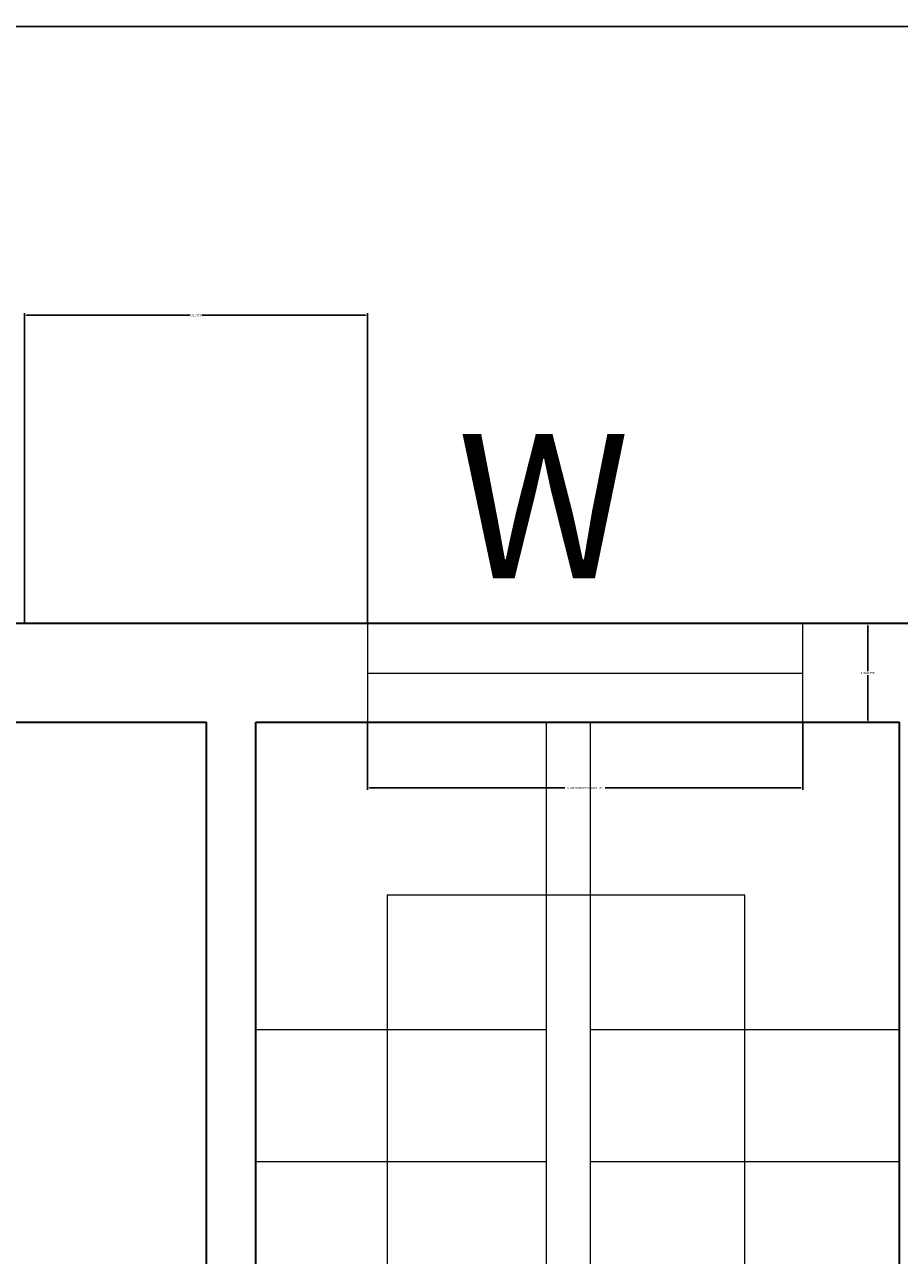
# Model space of a CAD drawing. Units: inches. Extents: x -26 to 788, y -42 to 505.
# Tile 7 of 9: x 219 to 298, y 374 to 486. Entities that reach past the tile are written whole.
import ezdxf

# ---------------------------------------------------------------- set-up
doc = ezdxf.new("R2010")
doc.units = ezdxf.units.IN
doc.header["$MEASUREMENT"] = 0
for name, color, linetype, lineweight in [('A-ANNO-DIMS', 2, 'Continuous', 18), ('A-ANNO-IDEN', 3, 'Continuous', 18), ('A-FLOR-STRS', 7, 'Continuous', 18), ('A-GLAZ', 4, 'Continuous', 18), ('A-WALL', 7, 'Continuous', 35)]:
    doc.layers.add(name, color=color, linetype=linetype, lineweight=lineweight)
doc.styles.get("Standard").update_dxf_attribs({"font": 'arial.ttf'})
doc.dimstyles.get("Standard").update_dxf_attribs({"dimtxt": 0.18, "dimasz": 0.18, "dimexe": 0.18, "dimexo": 0.0625, "dimgap": 0.09, "dimtad": 0, "dimtih": 1, "dimtoh": 1, "dimdec": 4, "dimzin": 0, "dimdsep": 46, "dimtxsty": 'Standard', "dimcen": 0.09, "dimadec": 0, "dimazin": 0, "dimtfac": 1, "dimtdec": 4, "dimtofl": 0, "dimtmove": 0, "dimatfit": 3, "dimfxl": 1, "dimtolj": 1, "dimtzin": 0, "dimarcsym": 0})

# ---------------------------------------------------------------- blocks, each defined once
blk = doc.blocks.new('*D7')
at = {"layer": 'A-ANNO-DIMS', "color": 0, "lineweight": -2, "transparency": 16777216}
for p, q in [((2.95, 431.18), (2.95, 485.53)), ((307.45, 431.18), (307.45, 485.53)), ((3.13, 485.35), (154.6, 485.35)), ((307.27, 485.35), (155.81, 485.35))]:
    blk.add_line(p, q, dxfattribs=at)
at = {"layer": 'A-ANNO-DIMS', "color": 0, "transparency": 16777216}
for points in [[(3.13, 485.38), (3.13, 485.32), (2.95, 485.35)], [(307.27, 485.38), (307.27, 485.32), (307.45, 485.35)]]:
    blk.add_solid(points, dxfattribs=at)
at = {"layer": 'Defpoints', "color": 0, "transparency": 16777216}
for p in [(307.45, 485.35), (2.95, 431.12), (307.45, 431.12)]:
    blk.add_point(p, dxfattribs=at)
at = {"layer": 'A-ANNO-DIMS', "color": 0, "transparency": 16777216, "insert": (155.2, 485.35), "char_height": 0.18, "attachment_point": 5}
blk.add_mtext('\\A1;304.5000', dxfattribs=at)
blk = doc.blocks.new('WIN-STAIR')
for p, q in [((0, 9), (0, 0)), ((39.57, 9), (39.57, 0)), ((0, 4.5), (39.58, 4.5))]:
    blk.add_line(p, q)
blk = doc.blocks.new('STAIR-RETURN')
for p, q in [((30.9, 12), (30.9, 123.91)), ((34.9, 0), (34.9, 123.91)), ((4.5, 96), (30.9, 96)), ((34.9, 96), (63, 96)), ((4.5, 84), (30.9, 84)), ((34.9, 84), (63, 84))]:
    blk.add_line(p, q)
blk.add_lwpolyline([(48.95, 36), (48.95, 108.21), (16.43, 108.21), (16.43, 53.45), (19.67, 56.58), (14.49, 56.53), (16.4, 53.46)])
blk = doc.blocks.new('*D31')
at = {"layer": 'A-ANNO-DIMS', "color": 0, "lineweight": -2, "transparency": 16777216}
for p, q in [((250.08, 422.02), (250.08, 415.97)), ((289.67, 422.02), (289.67, 415.97)), ((250.26, 416.15), (268.04, 416.15)), ((289.49, 416.15), (271.71, 416.15))]:
    blk.add_line(p, q, dxfattribs=at)
at = {"layer": 'A-ANNO-DIMS', "color": 0, "transparency": 16777216}
for points in [[(250.26, 416.18), (250.26, 416.12), (250.08, 416.15)], [(289.49, 416.18), (289.49, 416.12), (289.67, 416.15)]]:
    blk.add_solid(points, dxfattribs=at)
at = {"layer": 'Defpoints', "color": 0, "transparency": 16777216}
for p in [(250.08, 422.09), (289.67, 422.09), (289.67, 416.15)]:
    blk.add_point(p, dxfattribs=at)
at = {"layer": 'A-ANNO-DIMS', "color": 0, "transparency": 16777216, "insert": (269.88, 416.15), "char_height": 0.18, "attachment_point": 5}
blk.add_mtext('\\A1;STAIR WINDOW 39.5838 TYP.', dxfattribs=at)
blk = doc.blocks.new('*D32')
at = {"layer": 'A-ANNO-DIMS', "color": 0, "lineweight": -2, "transparency": 16777216}
for p, q in [((289.73, 431.09), (295.78, 431.09)), ((295.6, 430.91), (295.6, 426.77)), ((295.6, 422.27), (295.6, 426.4)), ((289.73, 422.09), (295.78, 422.09))]:
    blk.add_line(p, q, dxfattribs=at)
at = {"layer": 'A-ANNO-DIMS', "color": 0, "transparency": 16777216}
for points in [[(295.57, 430.91), (295.63, 430.91), (295.6, 431.09)], [(295.57, 422.27), (295.63, 422.27), (295.6, 422.09)]]:
    blk.add_solid(points, dxfattribs=at)
at = {"layer": 'Defpoints', "color": 0, "transparency": 16777216}
for p in [(289.67, 431.09), (295.6, 431.09), (289.67, 422.09)]:
    blk.add_point(p, dxfattribs=at)
at = {"layer": 'A-ANNO-DIMS', "color": 0, "transparency": 16777216, "insert": (295.6, 426.59), "char_height": 0.18, "attachment_point": 5}
blk.add_mtext('\\A1;9.0000 TYP.', dxfattribs=at)
blk = doc.blocks.new('*D55')
at = {"layer": 'A-ANNO-DIMS', "color": 0, "lineweight": -2, "transparency": 16777216}
for p, q in [((218.92, 431.23), (218.92, 459.29)), ((219.1, 459.11), (233.97, 459.11)), ((249.9, 459.11), (235.03, 459.11)), ((250.08, 431.15), (250.08, 459.29))]:
    blk.add_line(p, q, dxfattribs=at)
at = {"layer": 'A-ANNO-DIMS', "color": 0, "transparency": 16777216}
for points in [[(219.1, 459.14), (219.1, 459.08), (218.92, 459.11)], [(249.9, 459.14), (249.9, 459.08), (250.08, 459.11)]]:
    blk.add_solid(points, dxfattribs=at)
at = {"layer": 'Defpoints', "color": 0, "transparency": 16777216}
for p in [(250.08, 459.11), (218.92, 431.16), (250.08, 431.09)]:
    blk.add_point(p, dxfattribs=at)
at = {"layer": 'A-ANNO-DIMS', "color": 0, "transparency": 16777216, "insert": (234.5, 459.11), "char_height": 0.18, "attachment_point": 5}
blk.add_mtext('\\A1;31.1673', dxfattribs=at)

msp = doc.modelspace()

# ---------------------------------------------------------------- linework, layer by layer
at = {"layer": 'A-WALL'}
for p, q in [((2.95497, 431.11777), (307.45497, 431.11777)), ((128.95497, 422.11777), (235.45497, 422.11777)), ((235.45497, 310.20306), (235.45497, 422.11777)), ((239.95497, 310.20306), (239.95497, 422.11777)), ((239.95497, 422.11777), (298.45497, 422.11777)), ((298.45497, 164.11777), (298.45497, 422.11777))]:
    msp.add_line(p, q, dxfattribs=at)

# ---------------------------------------------------------------- block references
at = {"layer": 'A-FLOR-STRS'}
msp.add_blockref('STAIR-RETURN', (235.455, 298.203), dxfattribs=at)
at = {"layer": 'A-GLAZ'}
msp.add_blockref('WIN-STAIR', (250.083, 422.086), dxfattribs=at)

# ---------------------------------------------------------------- texts
at = {"layer": 'A-ANNO-IDEN'}
msp.add_text('W', height=13.09317, dxfattribs=at).set_placement((258.27152, 435.21429))

# ---------------------------------------------------------------- dimensions: what is measured, and where the dimension line sits
at = {"layer": 'A-ANNO-DIMS'}
for base, p1, p2, override, picture, middle in [((307.45497, 485.35153), (2.95497, 431.11777), (307.45497, 431.11777), {"dimclrd": 0, "dimclre": 0, "dimclrt": 0}, '*D7', (155.20497, 485.35153)), ((250.08341, 459.11412), (218.9161, 431.16412), (250.08341, 431.08567), {"dimdec": 4, "dimlfac": 1, "dimrnd": 0, "dimzin": 0, "dimdsep": 46, "dimlunit": 2}, '*D55', (234.49976, 459.11412))]:
    dim = msp.add_linear_dim(base=base, p1=p1, p2=p2, dimstyle='Standard', override=override, dxfattribs=at)
    dim.commit()
    dim.dimension.update_dxf_attribs({"geometry": picture, "text_midpoint": middle})
dim = msp.add_linear_dim(base=(295.60476, 431.08567), p1=(289.66719, 422.08567), p2=(289.66719, 431.08567), angle=90, text='<> TYP.', dimstyle='Standard', override={"dimdec": 4, "dimlfac": 1, "dimrnd": 0, "dimzin": 0, "dimdsep": 46, "dimlunit": 2}, dxfattribs=at)
dim.commit()
dim.dimension.update_dxf_attribs({"geometry": '*D32', "text_midpoint": (295.60476, 426.58567)})
dim = msp.add_linear_dim(base=(289.66719, 416.1481), p1=(250.08341, 422.08567), p2=(289.66719, 422.08567), text='STAIR WINDOW <> TYP.', dimstyle='Standard', override={"dimdec": 4, "dimlfac": 1, "dimrnd": 0, "dimzin": 0, "dimdsep": 46, "dimlunit": 2}, dxfattribs=at)
dim.commit()
dim.dimension.update_dxf_attribs({"geometry": '*D31', "text_midpoint": (269.8753, 416.1481)})

doc.saveas('drawing.dxf')
